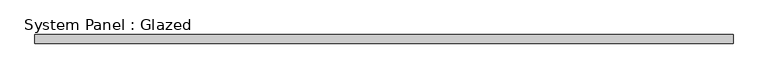
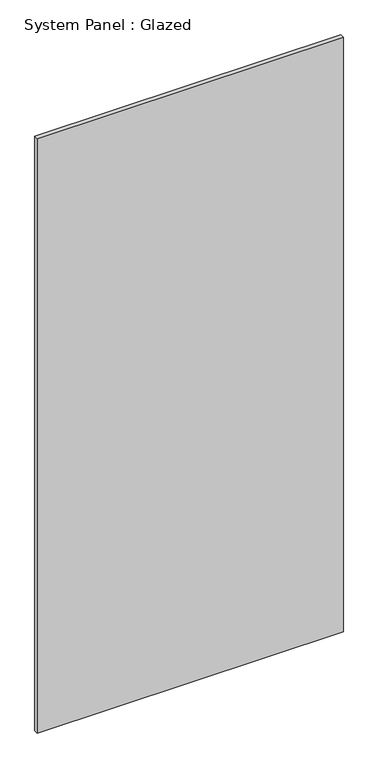
"""IFC4 building model written with IfcOpenShell, lengths in millimetres: plate geometry, System Panel : Glazed."""

from ifc_helpers import new_model, si_unit, origin, origin_with_axes, place, context, project, spatial, polyline, outline, extrude, source, transform, mapped, element, save


def system_panel_glazed_5cf703a3(model_context):
    return source(origin(), model_context, "Body", "SweptSolid", [
        extrude(outline(polyline([(975.0362552, 24.5), (-975.0362552, 24.5), (-975.0362552, 49.5), (975.0362552, 49.5), (975.0362552, 24.5)])), origin_with_axes(), (0.0, 0.0, 1.0), 4000.0),
    ])


if __name__ == "__main__":
    model = new_model("IFC4")
    model_context = context("Model", 3, world=origin())
    ifc_project = project(units=[si_unit("LENGTHUNIT", "METRE", prefix="MILLI")], contexts=[model_context])
    site = spatial("IfcSite", under=ifc_project)
    building = spatial("IfcBuilding", under=site)
    placement = place(None, origin())
    system_panel_glazed_shape = system_panel_glazed_5cf703a3(model_context)
    element("IfcPlate", 1, ObjectType="System Panel : Glazed", at=placement, inside=building, context=model_context, shape_type="MappedRepresentation", body=[
        mapped(system_panel_glazed_shape, transform((0.0, 0.0, 0.0), x_axis=(1.0, 0.0, 0.0), y_axis=(0.0, 1.0, 0.0), z_axis=(0.0, 0.0, 1.0))),
    ])
    save(model, "model.ifc")

# Revit data of these elements
# Type "System Panel : Glazed"
#   Keynote = "H11"
#   Construction Type Id = "GSP4R"
#   Analytic Construction = "1/8 in Pilkington single glazing"
#   Visual Light Transmittance = 0.9
#   Solar Heat Gain Coefficient = 0.86
#   Heat Transfer Coefficient (U) = 6.7069 W/(m²·K)
#   Define Thermal Properties by = 1
# Element 1 (IfcPlate, "System Panel : Glazed")
#   Materials on its faces: "Glass"
# Materials
#   "Glass": class "Glass", colour RGB 0 128 192, transparency 0.9, Description = "Soda Lime Glass", Cost = 0
